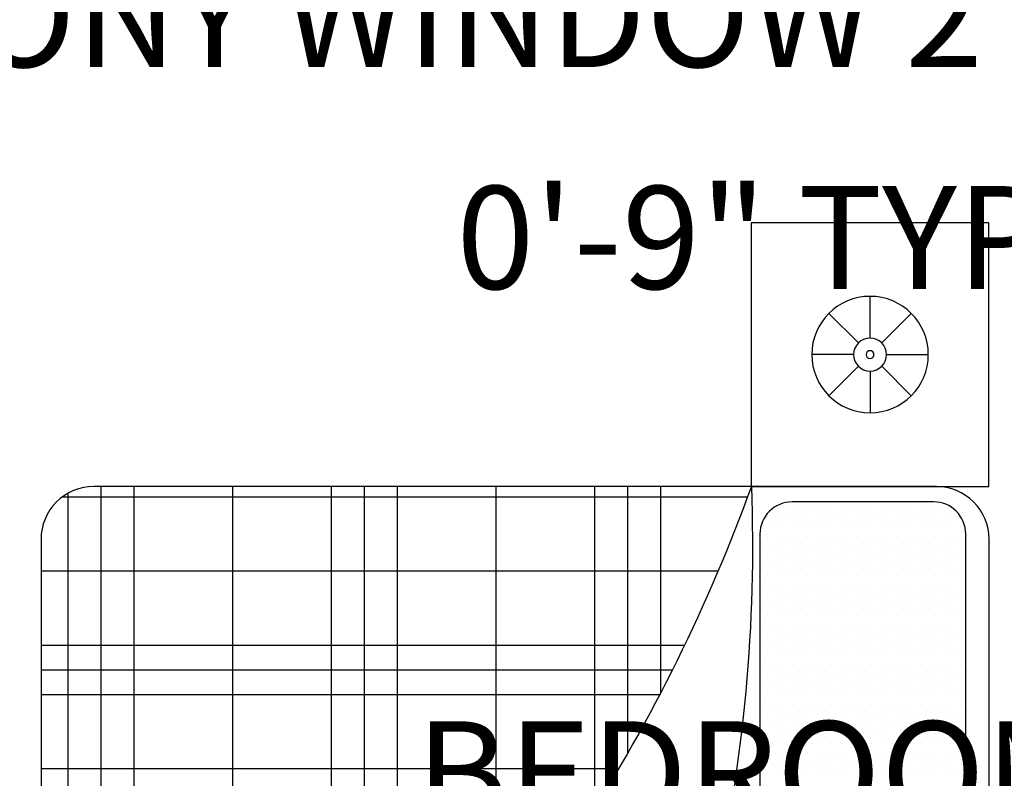
# Model space of a CAD drawing. Units: inches. Extents: x 528 to 2520, y -151 to 1354.
# Tile 24 of 41: x 1350 to 1407, y 1195 to 1239. Entities that reach past the tile are written whole.
import ezdxf

# ---------------------------------------------------------------- set-up
doc = ezdxf.new("R2010")
doc.units = ezdxf.units.IN
doc.header["$MEASUREMENT"] = 0
doc.layers.add('A-ANNO-DIMS', color=2, linetype='Continuous', lineweight=18)
doc.layers.add('A-FURN', color=8, linetype='Continuous', lineweight=18)
doc.layers.add('BLOCK', color=6, linetype='Continuous')
doc.styles.get("Standard").update_dxf_attribs({"font": 'arial.ttf'})
doc.dimstyles.get("Standard").update_dxf_attribs({"dimtxt": 6, "dimasz": 2, "dimexe": 0.18, "dimexo": 0.0625, "dimgap": 0.09, "dimtad": 0, "dimtih": 1, "dimtoh": 1, "dimdec": 1, "dimzin": 0, "dimdsep": 46, "dimlunit": 3, "dimtxsty": 'Standard', "dimblk": 'ARCHTICK', "dimcen": 0.09, "dimadec": 0, "dimazin": 0, "dimtfac": 1, "dimtdec": 1, "dimtofl": 0, "dimtmove": 0, "dimatfit": 3, "dimfxl": 1, "dimtolj": 1, "dimtzin": 0, "dimarcsym": 0})

# ---------------------------------------------------------------- blocks, each defined once
blk = doc.blocks.new('*X15')
at = {"color": 0}
for p, q in [((276.598, 451.25), (280.51, 451.25)), ((275.455, 450.625), (280.51, 450.625)), ((274.411, 450), (280.51, 450)), ((265.51, 448.125), (267.634, 448.125)), ((271.723, 448.125), (280.51, 448.125)), ((265.51, 446.25), (268.465, 446.25)), ((269.519, 446.25), (280.51, 446.25)), ((265.51, 445.625), (268.531, 445.625)), ((268.866, 445.625), (280.51, 445.625)), ((265.51, 445), (280.51, 445)), ((265.51, 443.125), (280.51, 443.125)), ((265.51, 441.25), (280.51, 441.25)), ((265.51, 440.625), (280.51, 440.625)), ((265.634, 440), (280.386, 440))]:
    blk.add_line(p, q, dxfattribs=at)
blk = doc.blocks.new('*X16')
at = {"color": 0}
for p, q in [((280.312, 439.886), (280.312, 452.896)), ((278.906, 439.482), (278.906, 452.338)), ((277.5, 439.482), (277.5, 451.702)), ((277.031, 439.482), (277.031, 451.471)), ((276.562, 439.482), (276.562, 451.231)), ((275.156, 439.482), (275.156, 450.451)), ((265.781, 439.797), (265.781, 449.511)), ((273.75, 439.482), (273.75, 449.576)), ((266.25, 439.517), (266.25, 449.296)), ((273.281, 439.482), (273.281, 449.261)), ((272.812, 439.482), (272.812, 448.934)), ((267.656, 439.482), (267.656, 448.095)), ((271.406, 439.482), (271.406, 447.876)), ((270, 439.482), (270, 446.689)), ((269.531, 439.482), (269.531, 446.262)), ((269.062, 439.482), (269.062, 445.817))]:
    blk.add_line(p, q, dxfattribs=at)
blk = doc.blocks.new('*X17')
at = {"color": 0}
for p, q in [((275.0625, 457.03125), (275.0625, 457.03125)), ((275.25, 456.9375), (275.25, 456.9375)), ((275.4375, 457.03125), (275.4375, 457.03125)), ((275.625, 456.9375), (275.625, 456.9375)), ((275.8125, 457.03125), (275.8125, 457.03125)), ((276, 456.9375), (276, 456.9375)), ((276.1875, 457.03125), (276.1875, 457.03125)), ((276.375, 456.9375), (276.375, 456.9375)), ((276.5625, 457.03125), (276.5625, 457.03125)), ((276.75, 456.9375), (276.75, 456.9375)), ((276.9375, 457.03125), (276.9375, 457.03125)), ((277.125, 456.9375), (277.125, 456.9375)), ((277.3125, 457.03125), (277.3125, 457.03125)), ((277.5, 456.9375), (277.5, 456.9375)), ((277.6875, 457.03125), (277.6875, 457.03125)), ((277.875, 456.9375), (277.875, 456.9375)), ((278.0625, 457.03125), (278.0625, 457.03125)), ((278.25, 456.9375), (278.25, 456.9375)), ((278.4375, 457.03125), (278.4375, 457.03125)), ((278.625, 456.9375), (278.625, 456.9375)), ((278.8125, 457.03125), (278.8125, 457.03125)), ((279, 456.9375), (279, 456.9375)), ((279.1875, 457.03125), (279.1875, 457.03125)), ((279.375, 456.9375), (279.375, 456.9375)), ((279.5625, 457.03125), (279.5625, 457.03125)), ((279.75, 456.9375), (279.75, 456.9375)), ((275.0625, 456.84375), (275.0625, 456.84375)), ((275.25, 456.75), (275.25, 456.75)), ((275.4375, 456.84375), (275.4375, 456.84375)), ((275.625, 456.75), (275.625, 456.75)), ((275.8125, 456.84375), (275.8125, 456.84375)), ((276, 456.75), (276, 456.75)), ((276.1875, 456.84375), (276.1875, 456.84375)), ((276.375, 456.75), (276.375, 456.75)), ((276.5625, 456.84375), (276.5625, 456.84375)), ((276.75, 456.75), (276.75, 456.75)), ((276.9375, 456.84375), (276.9375, 456.84375)), ((277.125, 456.75), (277.125, 456.75)), ((277.3125, 456.84375), (277.3125, 456.84375)), ((277.5, 456.75), (277.5, 456.75)), ((277.6875, 456.84375), (277.6875, 456.84375)), ((277.875, 456.75), (277.875, 456.75)), ((278.0625, 456.84375), (278.0625, 456.84375)), ((278.25, 456.75), (278.25, 456.75)), ((278.4375, 456.84375), (278.4375, 456.84375)), ((278.625, 456.75), (278.625, 456.75)), ((278.8125, 456.84375), (278.8125, 456.84375)), ((279, 456.75), (279, 456.75)), ((279.1875, 456.84375), (279.1875, 456.84375)), ((279.375, 456.75), (279.375, 456.75)), ((279.5625, 456.84375), (279.5625, 456.84375)), ((279.75, 456.75), (279.75, 456.75)), ((279.9375, 456.84375), (279.9375, 456.84375)), ((280.125, 456.75), (280.125, 456.75)), ((275.0625, 456.65625), (275.0625, 456.65625)), ((275.25, 456.5625), (275.25, 456.5625)), ((275.4375, 456.65625), (275.4375, 456.65625)), ((275.625, 456.5625), (275.625, 456.5625)), ((275.8125, 456.65625), (275.8125, 456.65625)), ((276, 456.5625), (276, 456.5625)), ((276.1875, 456.65625), (276.1875, 456.65625)), ((276.375, 456.5625), (276.375, 456.5625)), ((276.5625, 456.65625), (276.5625, 456.65625)), ((276.75, 456.5625), (276.75, 456.5625)), ((276.9375, 456.65625), (276.9375, 456.65625)), ((277.125, 456.5625), (277.125, 456.5625)), ((277.3125, 456.65625), (277.3125, 456.65625)), ((277.5, 456.5625), (277.5, 456.5625)), ((277.6875, 456.65625), (277.6875, 456.65625)), ((277.875, 456.5625), (277.875, 456.5625)), ((278.0625, 456.65625), (278.0625, 456.65625)), ((278.25, 456.5625), (278.25, 456.5625)), ((278.4375, 456.65625), (278.4375, 456.65625)), ((278.625, 456.5625), (278.625, 456.5625)), ((278.8125, 456.65625), (278.8125, 456.65625)), ((279, 456.5625), (279, 456.5625)), ((279.1875, 456.65625), (279.1875, 456.65625)), ((279.375, 456.5625), (279.375, 456.5625)), ((279.5625, 456.65625), (279.5625, 456.65625)), ((279.75, 456.5625), (279.75, 456.5625)), ((279.9375, 456.65625), (279.9375, 456.65625)), ((280.125, 456.5625), (280.125, 456.5625)), ((275.0625, 456.46875), (275.0625, 456.46875)), ((275.25, 456.375), (275.25, 456.375)), ((275.4375, 456.46875), (275.4375, 456.46875)), ((275.625, 456.375), (275.625, 456.375)), ((275.8125, 456.46875), (275.8125, 456.46875)), ((276, 456.375), (276, 456.375)), ((276.1875, 456.46875), (276.1875, 456.46875)), ((276.375, 456.375), (276.375, 456.375)), ((276.5625, 456.46875), (276.5625, 456.46875)), ((276.75, 456.375), (276.75, 456.375)), ((276.9375, 456.46875), (276.9375, 456.46875)), ((277.125, 456.375), (277.125, 456.375)), ((277.3125, 456.46875), (277.3125, 456.46875)), ((277.5, 456.375), (277.5, 456.375)), ((277.6875, 456.46875), (277.6875, 456.46875)), ((277.875, 456.375), (277.875, 456.375)), ((278.0625, 456.46875), (278.0625, 456.46875)), ((278.25, 456.375), (278.25, 456.375)), ((278.4375, 456.46875), (278.4375, 456.46875)), ((278.625, 456.375), (278.625, 456.375)), ((278.8125, 456.46875), (278.8125, 456.46875)), ((279, 456.375), (279, 456.375)), ((279.1875, 456.46875), (279.1875, 456.46875)), ((279.375, 456.375), (279.375, 456.375)), ((279.5625, 456.46875), (279.5625, 456.46875)), ((279.75, 456.375), (279.75, 456.375)), ((279.9375, 456.46875), (279.9375, 456.46875)), ((280.125, 456.375), (280.125, 456.375)), ((275.0625, 456.28125), (275.0625, 456.28125)), ((275.25, 456.1875), (275.25, 456.1875)), ((275.4375, 456.28125), (275.4375, 456.28125)), ((275.625, 456.1875), (275.625, 456.1875)), ((275.8125, 456.28125), (275.8125, 456.28125)), ((276, 456.1875), (276, 456.1875)), ((276.1875, 456.28125), (276.1875, 456.28125)), ((276.375, 456.1875), (276.375, 456.1875)), ((276.5625, 456.28125), (276.5625, 456.28125)), ((276.75, 456.1875), (276.75, 456.1875)), ((276.9375, 456.28125), (276.9375, 456.28125)), ((277.125, 456.1875), (277.125, 456.1875)), ((277.3125, 456.28125), (277.3125, 456.28125)), ((277.5, 456.1875), (277.5, 456.1875)), ((277.6875, 456.28125), (277.6875, 456.28125)), ((277.875, 456.1875), (277.875, 456.1875)), ((278.0625, 456.28125), (278.0625, 456.28125)), ((278.25, 456.1875), (278.25, 456.1875)), ((278.4375, 456.28125), (278.4375, 456.28125)), ((278.625, 456.1875), (278.625, 456.1875)), ((278.8125, 456.28125), (278.8125, 456.28125)), ((279, 456.1875), (279, 456.1875)), ((279.1875, 456.28125), (279.1875, 456.28125)), ((279.375, 456.1875), (279.375, 456.1875)), ((279.5625, 456.28125), (279.5625, 456.28125)), ((279.75, 456.1875), (279.75, 456.1875)), ((279.9375, 456.28125), (279.9375, 456.28125)), ((280.125, 456.1875), (280.125, 456.1875)), ((275.0625, 456.09375), (275.0625, 456.09375)), ((275.25, 456), (275.25, 456)), ((275.4375, 456.09375), (275.4375, 456.09375)), ((275.625, 456), (275.625, 456)), ((275.8125, 456.09375), (275.8125, 456.09375)), ((276, 456), (276, 456)), ((276.1875, 456.09375), (276.1875, 456.09375)), ((276.375, 456), (276.375, 456)), ((276.5625, 456.09375), (276.5625, 456.09375)), ((276.75, 456), (276.75, 456)), ((276.9375, 456.09375), (276.9375, 456.09375)), ((277.125, 456), (277.125, 456)), ((277.3125, 456.09375), (277.3125, 456.09375)), ((277.5, 456), (277.5, 456)), ((277.6875, 456.09375), (277.6875, 456.09375)), ((277.875, 456), (277.875, 456)), ((278.0625, 456.09375), (278.0625, 456.09375)), ((278.25, 456), (278.25, 456)), ((278.4375, 456.09375), (278.4375, 456.09375)), ((278.625, 456), (278.625, 456)), ((278.8125, 456.09375), (278.8125, 456.09375)), ((279, 456), (279, 456)), ((279.1875, 456.09375), (279.1875, 456.09375)), ((279.375, 456), (279.375, 456)), ((279.5625, 456.09375), (279.5625, 456.09375)), ((279.75, 456), (279.75, 456)), ((279.9375, 456.09375), (279.9375, 456.09375)), ((280.125, 456), (280.125, 456)), ((275.0625, 455.90625), (275.0625, 455.90625)), ((275.25, 455.8125), (275.25, 455.8125)), ((275.4375, 455.90625), (275.4375, 455.90625)), ((275.625, 455.8125), (275.625, 455.8125)), ((275.8125, 455.90625), (275.8125, 455.90625)), ((276, 455.8125), (276, 455.8125)), ((276.1875, 455.90625), (276.1875, 455.90625)), ((276.375, 455.8125), (276.375, 455.8125)), ((276.5625, 455.90625), (276.5625, 455.90625)), ((276.75, 455.8125), (276.75, 455.8125)), ((276.9375, 455.90625), (276.9375, 455.90625)), ((277.125, 455.8125), (277.125, 455.8125)), ((277.3125, 455.90625), (277.3125, 455.90625)), ((277.5, 455.8125), (277.5, 455.8125)), ((277.6875, 455.90625), (277.6875, 455.90625)), ((277.875, 455.8125), (277.875, 455.8125)), ((278.0625, 455.90625), (278.0625, 455.90625)), ((278.25, 455.8125), (278.25, 455.8125)), ((278.4375, 455.90625), (278.4375, 455.90625)), ((278.625, 455.8125), (278.625, 455.8125)), ((278.8125, 455.90625), (278.8125, 455.90625)), ((279, 455.8125), (279, 455.8125)), ((279.1875, 455.90625), (279.1875, 455.90625)), ((279.375, 455.8125), (279.375, 455.8125)), ((279.5625, 455.90625), (279.5625, 455.90625)), ((279.75, 455.8125), (279.75, 455.8125)), ((279.9375, 455.90625), (279.9375, 455.90625)), ((280.125, 455.8125), (280.125, 455.8125)), ((275.0625, 455.71875), (275.0625, 455.71875)), ((275.25, 455.625), (275.25, 455.625)), ((275.4375, 455.71875), (275.4375, 455.71875)), ((275.625, 455.625), (275.625, 455.625)), ((275.8125, 455.71875), (275.8125, 455.71875)), ((276, 455.625), (276, 455.625)), ((276.1875, 455.71875), (276.1875, 455.71875)), ((276.375, 455.625), (276.375, 455.625)), ((276.5625, 455.71875), (276.5625, 455.71875)), ((276.75, 455.625), (276.75, 455.625)), ((276.9375, 455.71875), (276.9375, 455.71875)), ((277.125, 455.625), (277.125, 455.625)), ((277.3125, 455.71875), (277.3125, 455.71875)), ((277.5, 455.625), (277.5, 455.625)), ((277.6875, 455.71875), (277.6875, 455.71875)), ((277.875, 455.625), (277.875, 455.625)), ((278.0625, 455.71875), (278.0625, 455.71875)), ((278.25, 455.625), (278.25, 455.625)), ((278.4375, 455.71875), (278.4375, 455.71875)), ((278.625, 455.625), (278.625, 455.625)), ((278.8125, 455.71875), (278.8125, 455.71875)), ((279, 455.625), (279, 455.625)), ((279.1875, 455.71875), (279.1875, 455.71875)), ((279.375, 455.625), (279.375, 455.625)), ((279.5625, 455.71875), (279.5625, 455.71875)), ((279.75, 455.625), (279.75, 455.625)), ((279.9375, 455.71875), (279.9375, 455.71875)), ((280.125, 455.625), (280.125, 455.625)), ((275.0625, 455.53125), (275.0625, 455.53125)), ((275.25, 455.4375), (275.25, 455.4375)), ((275.4375, 455.53125), (275.4375, 455.53125)), ((275.625, 455.4375), (275.625, 455.4375)), ((275.8125, 455.53125), (275.8125, 455.53125)), ((276, 455.4375), (276, 455.4375)), ((276.1875, 455.53125), (276.1875, 455.53125)), ((276.375, 455.4375), (276.375, 455.4375)), ((276.5625, 455.53125), (276.5625, 455.53125)), ((276.75, 455.4375), (276.75, 455.4375)), ((276.9375, 455.53125), (276.9375, 455.53125)), ((277.125, 455.4375), (277.125, 455.4375)), ((277.3125, 455.53125), (277.3125, 455.53125)), ((277.5, 455.4375), (277.5, 455.4375)), ((277.6875, 455.53125), (277.6875, 455.53125)), ((277.875, 455.4375), (277.875, 455.4375)), ((278.0625, 455.53125), (278.0625, 455.53125)), ((278.25, 455.4375), (278.25, 455.4375)), ((278.4375, 455.53125), (278.4375, 455.53125)), ((278.625, 455.4375), (278.625, 455.4375)), ((278.8125, 455.53125), (278.8125, 455.53125)), ((279, 455.4375), (279, 455.4375)), ((279.1875, 455.53125), (279.1875, 455.53125)), ((279.375, 455.4375), (279.375, 455.4375)), ((279.5625, 455.53125), (279.5625, 455.53125)), ((279.75, 455.4375), (279.75, 455.4375)), ((279.9375, 455.53125), (279.9375, 455.53125)), ((280.125, 455.4375), (280.125, 455.4375)), ((275.0625, 455.34375), (275.0625, 455.34375)), ((275.25, 455.25), (275.25, 455.25)), ((275.4375, 455.34375), (275.4375, 455.34375)), ((275.625, 455.25), (275.625, 455.25)), ((275.8125, 455.34375), (275.8125, 455.34375)), ((276, 455.25), (276, 455.25)), ((276.1875, 455.34375), (276.1875, 455.34375)), ((276.375, 455.25), (276.375, 455.25)), ((276.5625, 455.34375), (276.5625, 455.34375)), ((276.75, 455.25), (276.75, 455.25)), ((276.9375, 455.34375), (276.9375, 455.34375)), ((277.125, 455.25), (277.125, 455.25)), ((277.3125, 455.34375), (277.3125, 455.34375)), ((277.5, 455.25), (277.5, 455.25)), ((277.6875, 455.34375), (277.6875, 455.34375)), ((277.875, 455.25), (277.875, 455.25)), ((278.0625, 455.34375), (278.0625, 455.34375)), ((278.25, 455.25), (278.25, 455.25)), ((278.4375, 455.34375), (278.4375, 455.34375)), ((278.625, 455.25), (278.625, 455.25)), ((278.8125, 455.34375), (278.8125, 455.34375)), ((279, 455.25), (279, 455.25)), ((279.1875, 455.34375), (279.1875, 455.34375)), ((279.375, 455.25), (279.375, 455.25)), ((279.5625, 455.34375), (279.5625, 455.34375)), ((279.75, 455.25), (279.75, 455.25)), ((279.9375, 455.34375), (279.9375, 455.34375)), ((280.125, 455.25), (280.125, 455.25)), ((275.0625, 455.15625), (275.0625, 455.15625)), ((275.25, 455.0625), (275.25, 455.0625)), ((275.4375, 455.15625), (275.4375, 455.15625)), ((275.625, 455.0625), (275.625, 455.0625)), ((275.8125, 455.15625), (275.8125, 455.15625)), ((276, 455.0625), (276, 455.0625)), ((276.1875, 455.15625), (276.1875, 455.15625)), ((276.375, 455.0625), (276.375, 455.0625)), ((276.5625, 455.15625), (276.5625, 455.15625)), ((276.75, 455.0625), (276.75, 455.0625)), ((276.9375, 455.15625), (276.9375, 455.15625)), ((277.125, 455.0625), (277.125, 455.0625)), ((277.3125, 455.15625), (277.3125, 455.15625)), ((277.5, 455.0625), (277.5, 455.0625)), ((277.6875, 455.15625), (277.6875, 455.15625)), ((277.875, 455.0625), (277.875, 455.0625)), ((278.0625, 455.15625), (278.0625, 455.15625)), ((278.25, 455.0625), (278.25, 455.0625)), ((278.4375, 455.15625), (278.4375, 455.15625)), ((278.625, 455.0625), (278.625, 455.0625)), ((278.8125, 455.15625), (278.8125, 455.15625)), ((279, 455.0625), (279, 455.0625)), ((279.1875, 455.15625), (279.1875, 455.15625)), ((279.375, 455.0625), (279.375, 455.0625)), ((279.5625, 455.15625), (279.5625, 455.15625)), ((279.75, 455.0625), (279.75, 455.0625)), ((279.9375, 455.15625), (279.9375, 455.15625)), ((280.125, 455.0625), (280.125, 455.0625)), ((275.0625, 454.96875), (275.0625, 454.96875)), ((275.25, 454.875), (275.25, 454.875)), ((275.4375, 454.96875), (275.4375, 454.96875)), ((275.625, 454.875), (275.625, 454.875)), ((275.8125, 454.96875), (275.8125, 454.96875)), ((276, 454.875), (276, 454.875)), ((276.1875, 454.96875), (276.1875, 454.96875)), ((276.375, 454.875), (276.375, 454.875)), ((276.5625, 454.96875), (276.5625, 454.96875)), ((276.75, 454.875), (276.75, 454.875)), ((276.9375, 454.96875), (276.9375, 454.96875)), ((277.125, 454.875), (277.125, 454.875)), ((277.3125, 454.96875), (277.3125, 454.96875)), ((277.5, 454.875), (277.5, 454.875)), ((277.6875, 454.96875), (277.6875, 454.96875)), ((277.875, 454.875), (277.875, 454.875)), ((278.0625, 454.96875), (278.0625, 454.96875)), ((278.25, 454.875), (278.25, 454.875)), ((278.4375, 454.96875), (278.4375, 454.96875)), ((278.625, 454.875), (278.625, 454.875)), ((278.8125, 454.96875), (278.8125, 454.96875)), ((279, 454.875), (279, 454.875)), ((279.1875, 454.96875), (279.1875, 454.96875)), ((279.375, 454.875), (279.375, 454.875)), ((279.5625, 454.96875), (279.5625, 454.96875)), ((279.75, 454.875), (279.75, 454.875)), ((279.9375, 454.96875), (279.9375, 454.96875)), ((280.125, 454.875), (280.125, 454.875)), ((275.0625, 454.78125), (275.0625, 454.78125)), ((275.25, 454.6875), (275.25, 454.6875)), ((275.4375, 454.78125), (275.4375, 454.78125)), ((275.625, 454.6875), (275.625, 454.6875)), ((275.8125, 454.78125), (275.8125, 454.78125)), ((276, 454.6875), (276, 454.6875)), ((276.1875, 454.78125), (276.1875, 454.78125)), ((276.375, 454.6875), (276.375, 454.6875)), ((276.5625, 454.78125), (276.5625, 454.78125)), ((276.75, 454.6875), (276.75, 454.6875)), ((276.9375, 454.78125), (276.9375, 454.78125)), ((277.125, 454.6875), (277.125, 454.6875)), ((277.3125, 454.78125), (277.3125, 454.78125)), ((277.5, 454.6875), (277.5, 454.6875)), ((277.6875, 454.78125), (277.6875, 454.78125)), ((277.875, 454.6875), (277.875, 454.6875)), ((278.0625, 454.78125), (278.0625, 454.78125)), ((278.25, 454.6875), (278.25, 454.6875)), ((278.4375, 454.78125), (278.4375, 454.78125)), ((278.625, 454.6875), (278.625, 454.6875)), ((278.8125, 454.78125), (278.8125, 454.78125)), ((279, 454.6875), (279, 454.6875)), ((279.1875, 454.78125), (279.1875, 454.78125)), ((279.375, 454.6875), (279.375, 454.6875)), ((279.5625, 454.78125), (279.5625, 454.78125)), ((279.75, 454.6875), (279.75, 454.6875)), ((279.9375, 454.78125), (279.9375, 454.78125)), ((280.125, 454.6875), (280.125, 454.6875)), ((275.0625, 454.59375), (275.0625, 454.59375)), ((275.25, 454.5), (275.25, 454.5)), ((275.4375, 454.59375), (275.4375, 454.59375)), ((275.625, 454.5), (275.625, 454.5)), ((275.8125, 454.59375), (275.8125, 454.59375)), ((276, 454.5), (276, 454.5)), ((276.1875, 454.59375), (276.1875, 454.59375)), ((276.375, 454.5), (276.375, 454.5)), ((276.5625, 454.59375), (276.5625, 454.59375)), ((276.75, 454.5), (276.75, 454.5)), ((276.9375, 454.59375), (276.9375, 454.59375)), ((277.125, 454.5), (277.125, 454.5)), ((277.3125, 454.59375), (277.3125, 454.59375)), ((277.5, 454.5), (277.5, 454.5)), ((277.6875, 454.59375), (277.6875, 454.59375)), ((277.875, 454.5), (277.875, 454.5)), ((278.0625, 454.59375), (278.0625, 454.59375)), ((278.25, 454.5), (278.25, 454.5)), ((278.4375, 454.59375), (278.4375, 454.59375)), ((278.625, 454.5), (278.625, 454.5)), ((278.8125, 454.59375), (278.8125, 454.59375)), ((279, 454.5), (279, 454.5)), ((279.1875, 454.59375), (279.1875, 454.59375)), ((279.375, 454.5), (279.375, 454.5)), ((279.5625, 454.59375), (279.5625, 454.59375)), ((279.75, 454.5), (279.75, 454.5)), ((279.9375, 454.59375), (279.9375, 454.59375)), ((280.125, 454.5), (280.125, 454.5)), ((275.0625, 454.40625), (275.0625, 454.40625)), ((275.25, 454.3125), (275.25, 454.3125)), ((275.4375, 454.40625), (275.4375, 454.40625)), ((275.625, 454.3125), (275.625, 454.3125)), ((275.8125, 454.40625), (275.8125, 454.40625)), ((276, 454.3125), (276, 454.3125)), ((276.1875, 454.40625), (276.1875, 454.40625)), ((276.375, 454.3125), (276.375, 454.3125)), ((276.5625, 454.40625), (276.5625, 454.40625)), ((276.75, 454.3125), (276.75, 454.3125)), ((276.9375, 454.40625), (276.9375, 454.40625)), ((277.125, 454.3125), (277.125, 454.3125)), ((277.3125, 454.40625), (277.3125, 454.40625)), ((277.5, 454.3125), (277.5, 454.3125)), ((277.6875, 454.40625), (277.6875, 454.40625)), ((277.875, 454.3125), (277.875, 454.3125)), ((278.0625, 454.40625), (278.0625, 454.40625)), ((278.25, 454.3125), (278.25, 454.3125)), ((278.4375, 454.40625), (278.4375, 454.40625)), ((278.625, 454.3125), (278.625, 454.3125)), ((278.8125, 454.40625), (278.8125, 454.40625)), ((279, 454.3125), (279, 454.3125)), ((279.1875, 454.40625), (279.1875, 454.40625)), ((279.375, 454.3125), (279.375, 454.3125)), ((279.5625, 454.40625), (279.5625, 454.40625)), ((279.75, 454.3125), (279.75, 454.3125)), ((279.9375, 454.40625), (279.9375, 454.40625)), ((280.125, 454.3125), (280.125, 454.3125)), ((275.0625, 454.21875), (275.0625, 454.21875)), ((275.25, 454.125), (275.25, 454.125)), ((275.4375, 454.21875), (275.4375, 454.21875)), ((275.625, 454.125), (275.625, 454.125)), ((275.8125, 454.21875), (275.8125, 454.21875)), ((276, 454.125), (276, 454.125)), ((276.1875, 454.21875), (276.1875, 454.21875)), ((276.375, 454.125), (276.375, 454.125)), ((276.5625, 454.21875), (276.5625, 454.21875)), ((276.75, 454.125), (276.75, 454.125)), ((276.9375, 454.21875), (276.9375, 454.21875)), ((277.125, 454.125), (277.125, 454.125)), ((277.3125, 454.21875), (277.3125, 454.21875)), ((277.5, 454.125), (277.5, 454.125)), ((277.6875, 454.21875), (277.6875, 454.21875)), ((277.875, 454.125), (277.875, 454.125)), ((278.0625, 454.21875), (278.0625, 454.21875)), ((278.25, 454.125), (278.25, 454.125)), ((278.4375, 454.21875), (278.4375, 454.21875)), ((278.625, 454.125), (278.625, 454.125)), ((278.8125, 454.21875), (278.8125, 454.21875)), ((279, 454.125), (279, 454.125)), ((279.1875, 454.21875), (279.1875, 454.21875)), ((279.375, 454.125), (279.375, 454.125)), ((279.5625, 454.21875), (279.5625, 454.21875)), ((279.75, 454.125), (279.75, 454.125)), ((279.9375, 454.21875), (279.9375, 454.21875)), ((280.125, 454.125), (280.125, 454.125)), ((275.0625, 454.03125), (275.0625, 454.03125)), ((275.25, 453.9375), (275.25, 453.9375)), ((275.4375, 454.03125), (275.4375, 454.03125)), ((275.625, 453.9375), (275.625, 453.9375)), ((275.8125, 454.03125), (275.8125, 454.03125)), ((276, 453.9375), (276, 453.9375)), ((276.1875, 454.03125), (276.1875, 454.03125)), ((276.375, 453.9375), (276.375, 453.9375)), ((276.5625, 454.03125), (276.5625, 454.03125)), ((276.75, 453.9375), (276.75, 453.9375)), ((276.9375, 454.03125), (276.9375, 454.03125)), ((277.125, 453.9375), (277.125, 453.9375)), ((277.3125, 454.03125), (277.3125, 454.03125)), ((277.5, 453.9375), (277.5, 453.9375)), ((277.6875, 454.03125), (277.6875, 454.03125)), ((277.875, 453.9375), (277.875, 453.9375)), ((278.0625, 454.03125), (278.0625, 454.03125)), ((278.25, 453.9375), (278.25, 453.9375)), ((278.4375, 454.03125), (278.4375, 454.03125)), ((278.625, 453.9375), (278.625, 453.9375)), ((278.8125, 454.03125), (278.8125, 454.03125)), ((279, 453.9375), (279, 453.9375)), ((279.1875, 454.03125), (279.1875, 454.03125)), ((279.375, 453.9375), (279.375, 453.9375)), ((279.5625, 454.03125), (279.5625, 454.03125)), ((279.75, 453.9375), (279.75, 453.9375)), ((279.9375, 454.03125), (279.9375, 454.03125)), ((280.125, 453.9375), (280.125, 453.9375)), ((275.0625, 453.84375), (275.0625, 453.84375)), ((275.25, 453.75), (275.25, 453.75)), ((275.4375, 453.84375), (275.4375, 453.84375)), ((275.625, 453.75), (275.625, 453.75)), ((275.8125, 453.84375), (275.8125, 453.84375)), ((276, 453.75), (276, 453.75)), ((276.1875, 453.84375), (276.1875, 453.84375)), ((276.375, 453.75), (276.375, 453.75)), ((276.5625, 453.84375), (276.5625, 453.84375)), ((276.75, 453.75), (276.75, 453.75)), ((276.9375, 453.84375), (276.9375, 453.84375)), ((277.125, 453.75), (277.125, 453.75)), ((277.3125, 453.84375), (277.3125, 453.84375)), ((277.5, 453.75), (277.5, 453.75)), ((277.6875, 453.84375), (277.6875, 453.84375)), ((277.875, 453.75), (277.875, 453.75)), ((278.0625, 453.84375), (278.0625, 453.84375)), ((278.25, 453.75), (278.25, 453.75)), ((278.4375, 453.84375), (278.4375, 453.84375)), ((278.625, 453.75), (278.625, 453.75)), ((278.8125, 453.84375), (278.8125, 453.84375)), ((279, 453.75), (279, 453.75)), ((279.1875, 453.84375), (279.1875, 453.84375)), ((279.375, 453.75), (279.375, 453.75)), ((279.5625, 453.84375), (279.5625, 453.84375)), ((279.75, 453.75), (279.75, 453.75)), ((279.9375, 453.84375), (279.9375, 453.84375)), ((280.125, 453.75), (280.125, 453.75)), ((275.0625, 453.65625), (275.0625, 453.65625)), ((275.25, 453.5625), (275.25, 453.5625)), ((275.4375, 453.65625), (275.4375, 453.65625)), ((275.625, 453.5625), (275.625, 453.5625)), ((275.8125, 453.65625), (275.8125, 453.65625)), ((276, 453.5625), (276, 453.5625)), ((276.1875, 453.65625), (276.1875, 453.65625)), ((276.375, 453.5625), (276.375, 453.5625)), ((276.5625, 453.65625), (276.5625, 453.65625)), ((276.75, 453.5625), (276.75, 453.5625)), ((276.9375, 453.65625), (276.9375, 453.65625)), ((277.125, 453.5625), (277.125, 453.5625)), ((277.3125, 453.65625), (277.3125, 453.65625)), ((277.5, 453.5625), (277.5, 453.5625)), ((277.6875, 453.65625), (277.6875, 453.65625)), ((277.875, 453.5625), (277.875, 453.5625)), ((278.0625, 453.65625), (278.0625, 453.65625)), ((278.25, 453.5625), (278.25, 453.5625)), ((278.4375, 453.65625), (278.4375, 453.65625)), ((278.625, 453.5625), (278.625, 453.5625)), ((278.8125, 453.65625), (278.8125, 453.65625)), ((279, 453.5625), (279, 453.5625)), ((279.1875, 453.65625), (279.1875, 453.65625)), ((279.375, 453.5625), (279.375, 453.5625)), ((279.5625, 453.65625), (279.5625, 453.65625)), ((279.75, 453.5625), (279.75, 453.5625)), ((279.9375, 453.65625), (279.9375, 453.65625)), ((280.125, 453.5625), (280.125, 453.5625)), ((275.0625, 453.46875), (275.0625, 453.46875)), ((275.25, 453.375), (275.25, 453.375)), ((275.4375, 453.46875), (275.4375, 453.46875)), ((275.625, 453.375), (275.625, 453.375)), ((275.8125, 453.46875), (275.8125, 453.46875)), ((276, 453.375), (276, 453.375)), ((276.1875, 453.46875), (276.1875, 453.46875)), ((276.375, 453.375), (276.375, 453.375)), ((276.5625, 453.46875), (276.5625, 453.46875)), ((276.75, 453.375), (276.75, 453.375)), ((276.9375, 453.46875), (276.9375, 453.46875)), ((277.125, 453.375), (277.125, 453.375)), ((277.3125, 453.46875), (277.3125, 453.46875)), ((277.5, 453.375), (277.5, 453.375)), ((277.6875, 453.46875), (277.6875, 453.46875)), ((277.875, 453.375), (277.875, 453.375)), ((278.0625, 453.46875), (278.0625, 453.46875)), ((278.25, 453.375), (278.25, 453.375)), ((278.4375, 453.46875), (278.4375, 453.46875)), ((278.625, 453.375), (278.625, 453.375)), ((278.8125, 453.46875), (278.8125, 453.46875)), ((279, 453.375), (279, 453.375)), ((279.1875, 453.46875), (279.1875, 453.46875)), ((279.375, 453.375), (279.375, 453.375)), ((279.5625, 453.46875), (279.5625, 453.46875)), ((279.75, 453.375), (279.75, 453.375)), ((279.9375, 453.46875), (279.9375, 453.46875)), ((275.0625, 453.28125), (275.0625, 453.28125)), ((275.25, 453.1875), (275.25, 453.1875)), ((275.4375, 453.28125), (275.4375, 453.28125)), ((275.625, 453.1875), (275.625, 453.1875)), ((275.8125, 453.28125), (275.8125, 453.28125)), ((276, 453.1875), (276, 453.1875)), ((276.1875, 453.28125), (276.1875, 453.28125)), ((276.375, 453.1875), (276.375, 453.1875)), ((276.5625, 453.28125), (276.5625, 453.28125)), ((276.75, 453.1875), (276.75, 453.1875)), ((276.9375, 453.28125), (276.9375, 453.28125)), ((277.125, 453.1875), (277.125, 453.1875)), ((277.3125, 453.28125), (277.3125, 453.28125)), ((277.5, 453.1875), (277.5, 453.1875)), ((277.6875, 453.28125), (277.6875, 453.28125)), ((277.875, 453.1875), (277.875, 453.1875)), ((278.0625, 453.28125), (278.0625, 453.28125)), ((278.25, 453.1875), (278.25, 453.1875)), ((278.4375, 453.28125), (278.4375, 453.28125)), ((278.625, 453.1875), (278.625, 453.1875)), ((278.8125, 453.28125), (278.8125, 453.28125)), ((279, 453.1875), (279, 453.1875)), ((279.1875, 453.28125), (279.1875, 453.28125)), ((279.375, 453.1875), (279.375, 453.1875)), ((279.5625, 453.28125), (279.5625, 453.28125)), ((279.75, 453.1875), (279.75, 453.1875)), ((279.9375, 453.28125), (279.9375, 453.28125))]:
    blk.add_line(p, q, dxfattribs=at)
blk = doc.blocks.new('A$C52E67D0D')
at = {"layer": 'BLOCK'}
for p, q in [((2251.5, 1605.5), (2251.5, 1684.7)), ((2229.3, 1596.3), (2173.3, 1652.3)), ((2273.7, 1596.3), (2329.7, 1652.3)), ((2220.1, 1574.1), (2140.9, 1574.1)), ((2282.9, 1574.1), (2362.1, 1574.1)), ((2229.3, 1551.9), (2173.3, 1495.9)), ((2273.7, 1551.9), (2329.7, 1495.9)), ((2251.5, 1542.8), (2251.5, 1463.5))]:
    blk.add_line(p, q, dxfattribs=at)
for points in [[(1901, 0), (601, 0, -0.414214), (501, 100), (501, 1700, -0.414214), (601, 1800), (1901, 1800, -0.414214), (2001, 1700), (2001, 100, -0.414214)], [(1911, 1365.1), (1335, 1365.1, -0.414214), (1274.2, 1425.9), (1274.2, 1694.8, -0.414214), (1335, 1755.7), (1911, 1755.7, -0.414214), (1971.8, 1694.8), (1971.8, 1425.9, -0.414214)]]:
    blk.add_lwpolyline(points, format="xyb", close=True, dxfattribs=at)
blk.add_lwpolyline([(2001, 1348.6), (2001, 1799.6), (2502, 1799.6), (2502, 1348.6)], close=True, dxfattribs=at)
for radius in [110.6, 31.4, 7.46]:
    blk.add_circle((2251.5, 1574.1), radius, dxfattribs=at)
for centre, radius, start, end in [((1888.6, -1664.5), 3015.3, 87.8642, 117.4001), ((3101, -1685.8), 3227.7, 109.926, 135.3977)]:
    blk.add_arc(centre, radius, start, end, dxfattribs=at)
at = {"layer": 'BLOCK', "xscale": 100, "yscale": 100, "zscale": 100}
for name in ['*X17', '*X16', '*X15']:
    blk.add_blockref(name, (-26050, -43948.2), dxfattribs=at)
blk = doc.blocks.new('_ArchTick')
at = {"color": 0, "linetype": 'ByBlock', "const_width": 0.15}
blk.add_lwpolyline([(-0.5, -0.5), (0.5, 0.5)], dxfattribs=at)
blk = doc.blocks.new('*D44')
at = {"layer": 'A-ANNO-DIMS', "color": 0, "lineweight": -2, "transparency": 16777216}
for p, q in [((1422.946, 1219.369), (1430.263, 1219.369)), ((1430.083, 1219.369), (1430.083, 1198.563)), ((1430.083, 1171.369), (1430.083, 1192.174)), ((1422.946, 1171.369), (1430.263, 1171.369))]:
    blk.add_line(p, q, dxfattribs=at)
at = {"layer": 'Defpoints', "color": 0, "transparency": 16777216}
for p in [(1422.883, 1219.369), (1430.083, 1219.369), (1422.883, 1171.369)]:
    blk.add_point(p, dxfattribs=at)
at = {"layer": 'A-ANNO-DIMS', "color": 0, "lineweight": -2, "transparency": 16777216, "xscale": 2, "yscale": 2, "zscale": 2}
for p, rotation in [((1430.083, 1219.369), 90), ((1430.083, 1171.369), 270)]:
    blk.add_blockref('_ArchTick', p, dxfattribs=dict(at, rotation=rotation))
at = {"layer": 'A-ANNO-DIMS', "color": 0, "transparency": 16777216, "insert": (1430.083, 1195.369), "char_height": 6, "attachment_point": 5}
blk.add_mtext('\\A1;BEDROOM WINDOW 4\'-0" TYP.', dxfattribs=at)
blk = doc.blocks.new('*D45')
at = {"layer": 'A-ANNO-DIMS', "color": 0, "lineweight": -2, "transparency": 16777216}
for p, q in [((1413.883, 1226.569), (1411.883, 1226.569)), ((1413.883, 1219.431), (1413.883, 1226.749)), ((1422.883, 1226.569), (1413.883, 1226.569)), ((1422.883, 1219.431), (1422.883, 1226.749))]:
    blk.add_line(p, q, dxfattribs=at)
at = {"layer": 'Defpoints', "color": 0, "transparency": 16777216}
for p in [(1413.883, 1226.569), (1413.883, 1219.369), (1422.883, 1219.369)]:
    blk.add_point(p, dxfattribs=at)
at = {"layer": 'A-ANNO-DIMS', "color": 0, "lineweight": -2, "transparency": 16777216, "xscale": 2, "yscale": 2, "zscale": 2, "rotation": 180}
blk.add_blockref('_ArchTick', (1413.883, 1226.569), dxfattribs=at)
at = {"layer": 'A-ANNO-DIMS', "color": 0, "lineweight": -2, "transparency": 16777216, "xscale": 2, "yscale": 2, "zscale": 2}
blk.add_blockref('_ArchTick', (1422.883, 1226.569), dxfattribs=at)
at = {"layer": 'A-ANNO-DIMS', "color": 0, "transparency": 16777216, "insert": (1393.507, 1226.569), "char_height": 6, "attachment_point": 5}
blk.add_mtext('\\A1;0\'-9" TYP.', dxfattribs=at)
blk = doc.blocks.new('*D86')
at = {"layer": 'A-ANNO-DIMS', "color": 0, "lineweight": -2, "transparency": 16777216}
for p, q in [((1297.45, 1243.04), (1297.45, 1239.323)), ((1321.45, 1243.04), (1321.45, 1239.323)), ((1297.45, 1239.503), (1321.45, 1239.503)), ((1321.45, 1239.503), (1323.45, 1239.503))]:
    blk.add_line(p, q, dxfattribs=at)
at = {"layer": 'Defpoints', "color": 0, "transparency": 16777216}
for p in [(1297.45, 1243.103), (1321.45, 1243.103), (1321.45, 1239.503)]:
    blk.add_point(p, dxfattribs=at)
at = {"layer": 'A-ANNO-DIMS', "color": 0, "lineweight": -2, "transparency": 16777216, "xscale": 2, "yscale": 2, "zscale": 2, "rotation": 180}
blk.add_blockref('_ArchTick', (1297.45, 1239.503), dxfattribs=at)
at = {"layer": 'A-ANNO-DIMS', "color": 0, "lineweight": -2, "transparency": 16777216, "xscale": 2, "yscale": 2, "zscale": 2}
blk.add_blockref('_ArchTick', (1321.45, 1239.503), dxfattribs=at)
at = {"layer": 'A-ANNO-DIMS', "color": 0, "transparency": 16777216, "insert": (1382.441, 1239.503), "char_height": 6, "attachment_point": 5}
blk.add_mtext('\\A1;BALCONY WINDOW 2\'-0" TYP.', dxfattribs=at)

msp = doc.modelspace()

# ---------------------------------------------------------------- block references
at = {"layer": 'A-FURN', "xscale": -0.0306954436450662, "yscale": 0.0306954436450662, "zscale": 0.0306954436450662, "rotation": 270}
msp.add_blockref('A$C52E67D0D', (1350.988, 1150.631), dxfattribs=at)

# ---------------------------------------------------------------- dimensions: what is measured, and where the dimension line sits
at = {"layer": 'A-ANNO-DIMS'}
dim = msp.add_linear_dim(base=(1321.45, 1239.503), p1=(1297.45, 1243.103), p2=(1321.45, 1243.103), text='BALCONY WINDOW <> TYP.', dimstyle='Standard', override={"dimdec": 1, "dimlfac": 1, "dimrnd": 0, "dimzin": 1, "dimdsep": 46, "dimlunit": 4, "dimfrac": 2}, dxfattribs=at)
dim.commit()
dim.dimension.update_dxf_attribs({"geometry": '*D86', "text_midpoint": (1382.441, 1239.503)})
for base, p1, p2, angle, text, picture, middle in [((1413.883, 1226.569), (1422.883, 1219.369), (1413.883, 1219.369), 180, '<> TYP.', '*D45', (1393.507, 1226.569)), ((1430.083, 1219.369), (1422.883, 1171.369), (1422.883, 1219.369), 90, 'BEDROOM WINDOW <> TYP.', '*D44', (1430.083, 1195.369))]:
    dim = msp.add_linear_dim(base=base, p1=p1, p2=p2, angle=angle, text=text, dimstyle='Standard', override={"dimdec": 1, "dimlfac": 1, "dimrnd": 0, "dimzin": 1, "dimdsep": 46, "dimlunit": 4, "dimfrac": 2}, dxfattribs=at)
    dim.commit()
    dim.dimension.update_dxf_attribs({"geometry": picture, "text_midpoint": middle})

doc.saveas('drawing.dxf')
